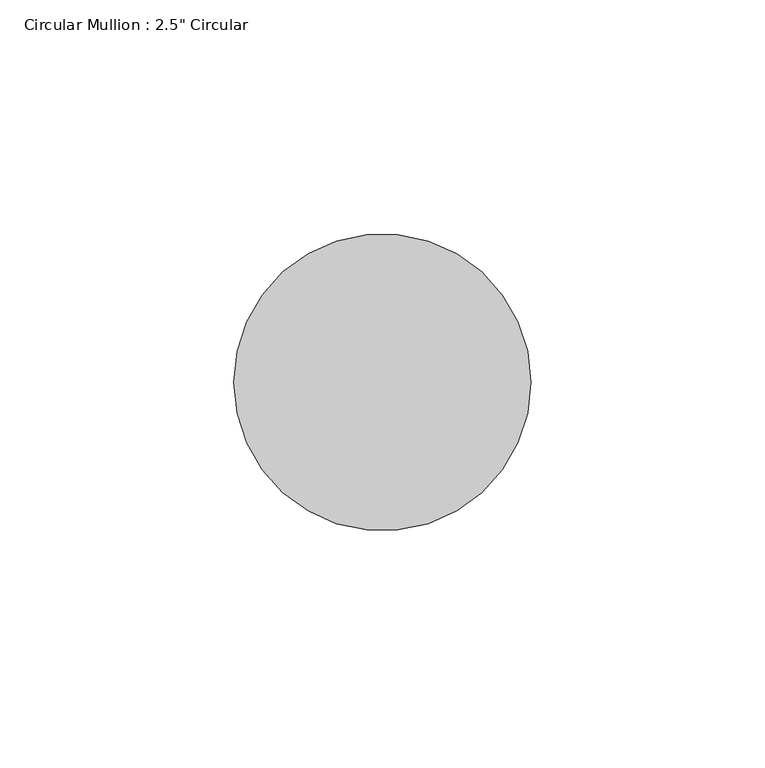
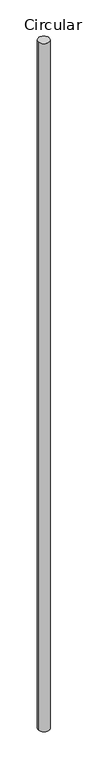
"""IFC4 building model written with IfcOpenShell, lengths in millimetres: member geometry."""

from ifc_helpers import new_model, si_unit, point, frame, frame_2d, origin, place, context, project, spatial, circle_curve, trimmed, segment, composite_curve, outline, extrude, source, transform, mapped, element, save


def member_62657261(model_context):
    return source(origin(), model_context, "Body", "SweptSolid", [
        extrude(outline(composite_curve([segment(trimmed(circle_curve(frame_2d((-31.75, 0.0)), 31.75), [point((0.0, 0.0))], [point((-63.5, 0.0))], False, "CARTESIAN"), True, "CONTINUOUS"), segment(trimmed(circle_curve(frame_2d((-31.75, 0.0)), 31.75), [point((-63.5, 0.0))], [point((0.0, 0.0))], False, "CARTESIAN"), True, "CONTINUOUS")], self_intersect=False)), frame((0.0, 0.0, -4114.8), z_axis=(0.0, 0.0, 1.0), x_axis=(1.0, 0.0, 0.0)), (0.0, 0.0, 1.0), 4114.8),
    ])


if __name__ == "__main__":
    model = new_model("IFC4")
    model_context = context("Model", 3, world=origin())
    ifc_project = project(units=[si_unit("LENGTHUNIT", "METRE", prefix="MILLI")], contexts=[model_context])
    site = spatial("IfcSite", under=ifc_project)
    building = spatial("IfcBuilding", under=site)
    placement = place(None, origin())
    member_shape = member_62657261(model_context)
    element("IfcMember", 1, ObjectType="Circular Mullion : 2.5\" Circular", at=placement, inside=building, context=model_context, shape_type="MappedRepresentation", body=[
        mapped(member_shape, transform((0.0, 0.0, 0.0), x_axis=(1.0, 0.0, 0.0), y_axis=(0.0, 1.0, 0.0), z_axis=(0.0, 0.0, 1.0))),
    ])
    save(model, "model.ifc")

# Revit data of these elements
# Type "Circular Mullion : 2.5\" Circular"
#   built-in parameter 1007350 = 0.104167 (stored number, unit not read)
# Element 1 (IfcMember, "Circular Mullion : 2.5\" Circular")
#   Materials on its faces: "Aluminum"
# Materials
#   "Aluminum": class "Metal", colour RGB 247 247 247, transparency 0, Description = "Aluminum 6061", Cost = 0
